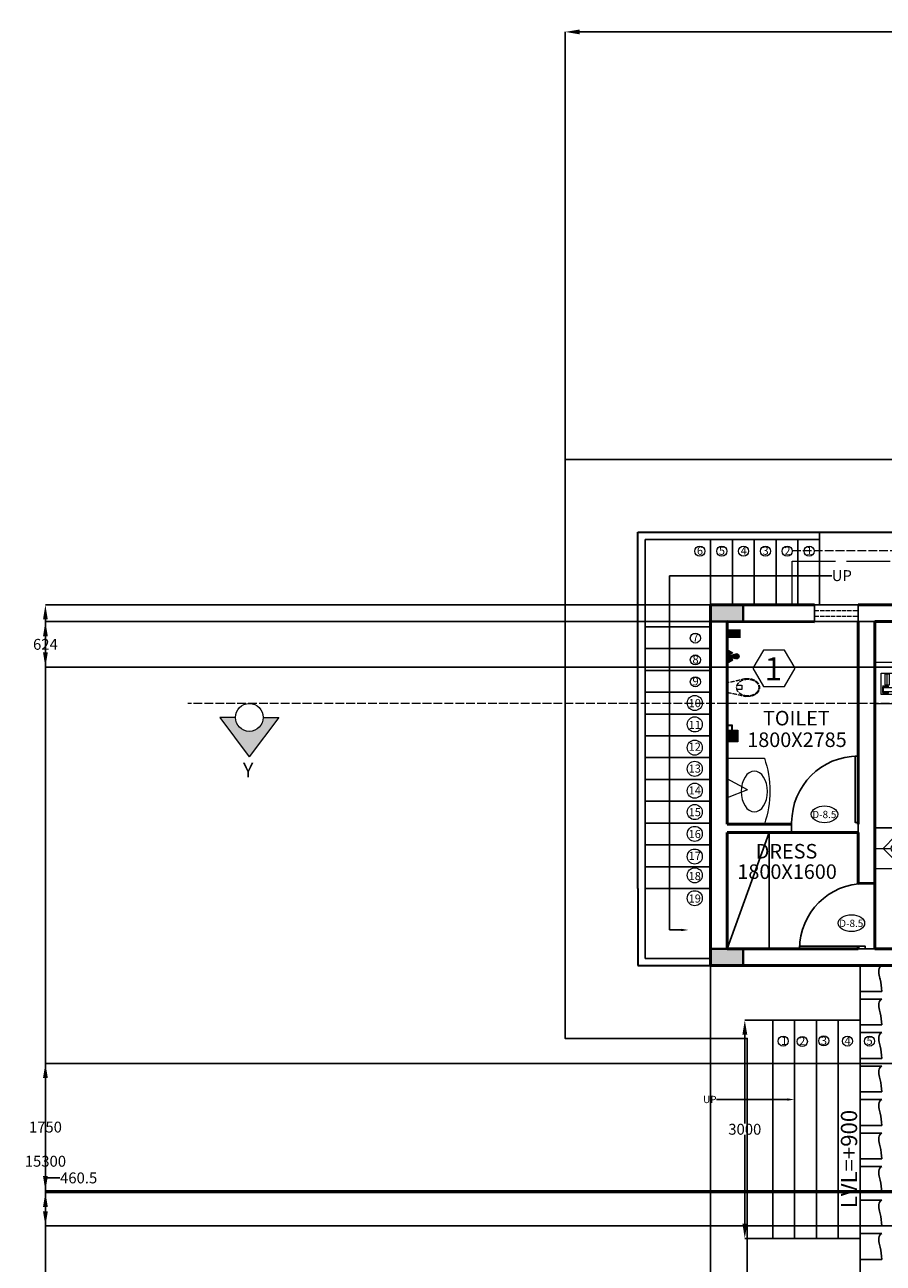
# Model space of a CAD drawing. Units: inches. Extents: x 22626 to 57351, y 2118 to 36234.
# Tile 2 of 10: x 22626 to 34432, y 19205 to 36234. Entities that reach past the tile are written whole.
import ezdxf
from ezdxf import colors
from ezdxf.entities.mleader import LeaderData, LeaderLine
from ezdxf.math import Vec2, Vec3

# ---------------------------------------------------------------- set-up
doc = ezdxf.new("R2010")
doc.units = ezdxf.units.IN
doc.header["$MEASUREMENT"] = 0
doc.linetypes.add('ACAD_ISO02W100', pattern=[15, 12, -3])
for name, color, linetype, lineweight in [('A-ANNO-DIMS', 130, 'Continuous', 18), ('A-ANNO-IDEN', 130, 'Continuous', 15), ('A-ANNO-STRS', 130, 'Continuous', 15), ('A-ANNO-SYMB', 130, 'Continuous', 18), ('A-AREA-IDEN', 130, 'Continuous', 18), ('A-COLS', 7, 'Continuous', 40), ('A-FLOR', 80, 'Continuous', 30), ('A-FLOR-CASE', 30, 'Continuous', 25), ('A-FLOR-FIXT', 30, 'Continuous', 18), ('A-FLOR-FIXT-HIDN', 30, 'ACAD_ISO02W100', 18), ('A-GLAZ-VENT', 152, 'Continuous', 25), ('A-GLAZ-VENT-HIDN', 152, 'ACAD_ISO02W100', 18), ('A-ROOF', 80, 'Continuous', 25), ('A-ROOF-OVHD', 80, 'ACAD_ISO02W100', 18), ('A-WALL', 80, 'Continuous', 50), ('DOORS', 32, 'Continuous', 25), ('FURNITURE', 30, 'Continuous', 18), ('STAIRS', 82, 'Continuous', 25)]:
    doc.layers.add(name, color=color, linetype=linetype, lineweight=lineweight)
doc.layers.add('A-SECT', color=2, linetype='ACAD_ISO02W100', lineweight=18, true_color=0xf1eb1f)
doc.styles.get("Standard").update_dxf_attribs({"font": 'arial.ttf'})
doc.dimstyles.get("Standard").update_dxf_attribs({"dimtxt": 150, "dimasz": 200, "dimexe": 0.18, "dimexo": 0.0625, "dimgap": 0.09, "dimtad": 0, "dimtih": 1, "dimtoh": 1, "dimdec": 0, "dimzin": 0, "dimdsep": 46, "dimtxsty": 'Standard', "dimcen": 0.09, "dimadec": 0, "dimazin": 0, "dimtfac": 1, "dimtdec": 0, "dimtofl": 0, "dimtmove": 0, "dimatfit": 3, "dimfxl": 1, "dimtolj": 1, "dimtzin": 0, "dimarcsym": 0})

# ---------------------------------------------------------------- blocks, each defined once
blk = doc.blocks.new('*U7')
for p, q in [((0, 0), (0, -6)), ((40, 0), (40, -6))]:
    blk.add_line(p, q)
blk.add_lwpolyline([(0, 0), (0, 40), (1.75, 40), (1.75, 0)], close=True)
blk.add_arc((0, 0), 40, 0, 90)
blk = doc.blocks.new('*D9')
at = {"layer": 'A-ANNO-DIMS', "color": 0, "lineweight": -2, "transparency": 16777216}
for p, q in [((32912, 22547), (32528, 22547)), ((32528, 22347), (32528, 21124)), ((32528, 19747), (32528, 20970)), ((32912, 19547), (32528, 19547))]:
    blk.add_line(p, q, dxfattribs=at)
at = {"layer": 'A-ANNO-DIMS', "color": 0, "transparency": 16777216}
for points in [[(32495, 22347), (32562, 22347), (32528, 22547)], [(32495, 19747), (32562, 19747), (32528, 19547)]]:
    blk.add_solid(points, dxfattribs=at)
at = {"layer": 'Defpoints', "color": 0, "transparency": 16777216}
for p in [(32912, 22547), (32528, 19547), (32912, 19547)]:
    blk.add_point(p, dxfattribs=at)
at = {"layer": 'A-ANNO-DIMS', "color": 0, "transparency": 16777216, "insert": (32528, 21047), "char_height": 150, "attachment_point": 5}
blk.add_mtext('\\A1;3000', dxfattribs=at)
blk = doc.blocks.new('Phone - Desk')
for p, q in [((-4.5, -5), (-4.5, 5)), ((-4.5, 5), (4.5, 5)), ((-4, 4.5), (-4, 2)), ((-4, 2), (-3.25, 2)), ((-3.75, 4.5), (-3.75, 2.25)), ((-1.25, 4.5), (-3.75, 4.5)), ((-3.75, 2.25), (-3.25, 2.25)), ((-3.25, 4), (-3.25, -4)), ((-3.25, 4), (-1.75, 4)), ((-1.75, -4), (-1.75, 4)), ((-1.75, 2.25), (-1.25, 2.25)), ((-1.75, 2), (-1, 2)), ((-1.25, 2.25), (-1.25, 4.5)), ((-1, 2), (-1, 4.5)), ((4, 3.5), (-0.5, 3.5)), ((-0.5, 3.5), (-0.5, 1.5)), ((-0.5, 2.5), (4, 2.5)), ((-0.5, 1.5), (4, 1.5)), ((4, 1.5), (4, 3.5)), ((4.5, 5), (4.5, -5)), ((4.5, -5), (-4.5, -5)), ((-3.75, -2.25), (-3.25, -2.25)), ((-3.75, -4.5), (-3.75, -2.25)), ((-1.25, -4.5), (-3.75, -4.5)), ((-3.25, -4), (-1.75, -4)), ((-1.75, -2.25), (-1.25, -2.25)), ((-1.25, -2.25), (-1.25, -4.5)), ((2.75, -1), (0.75, -1)), ((0.75, -1), (0.75, -4)), ((0.75, -4), (2.75, -4)), ((2.75, -4), (2.75, -1))]:
    blk.add_line(p, q)
blk = doc.blocks.new('BED')
h = blk.add_hatch()
h.set_pattern_fill('AR-B816', color=256, scale=27, angle=45)
h.paths.add_polyline_path([(36405, 26901), (36405, 25191), (35361, 25191), (35361, 24640), (36931, 24640), (36931, 25191), (36931, 27463), (36405, 27463), (35361, 27463), (35361, 26901)])
for p, q in [((35361, 26901), (35361, 27463)), ((35361, 27463), (36405, 27463)), ((36405, 27463), (36931, 27463)), ((36931, 27463), (36931, 25191)), ((35035, 26901), (35035, 26469)), ((34673, 25686), (34673, 26469)), ((35035, 26469), (34673, 26469)), ((35035, 25686), (34673, 25686)), ((34673, 25686), (35035, 25191)), ((35035, 25191), (35035, 25686)), ((34429, 24909), (34599, 25080)), ((34599, 25191), (34599, 24968)), ((34599, 25080), (34769, 24909)), ((35361, 24640), (35361, 25191)), ((36931, 25191), (36931, 24640)), ((34317, 24909), (34540, 24909)), ((34599, 24739), (34429, 24909)), ((34769, 24909), (34599, 24739)), ((34658, 24909), (34880, 24909)), ((34599, 24850), (34599, 24628)), ((36931, 24640), (35361, 24640))]:
    blk.add_line(p, q)
for points in [[(34317, 26901), (34880, 26901), (34880, 27463), (34317, 27463)], [(34317, 26901), (36405, 26901), (36405, 25191), (34317, 25191)], [(34317, 25191), (34880, 25191), (34880, 24628), (34317, 24628)]]:
    blk.add_lwpolyline(points, close=True)
blk.add_circle((34599, 24909), 59)
at = {"xscale": 32.52267765020765, "yscale": 32.52267765020765, "zscale": 32.52267765020765, "rotation": 90}
blk.add_blockref('Phone - Desk', (34567, 27173), dxfattribs=at)
blk = doc.blocks.new('WC')
at = {"ltscale": 5}
for p, q in [((307, 158), (242, 158)), ((242, 158), (242, 98)), ((242, 98), (310, 100)), ((307, 158), (307, 158))]:
    blk.add_line(p, q, dxfattribs=at)
for centre, start, end in [((781, 2286), 254.0006, 260.8285), ((781, -2036), 99.1715, 105.9994)]:
    blk.add_arc(centre, 2121, start, end, dxfattribs=at)
blk.add_ellipse((162, 125), major_axis=(152, 0), ratio=0.757128, start_param=-1.570796, end_param=4.712389, dxfattribs=at)
for points, knots in [([(196, 247), (190, 248), (184, 249), (169, 250), (159, 250), (141, 249), (132, 248), (115, 245), (106, 243), (89, 237), (81, 234), (66, 226), (59, 222), (45, 212), (39, 207), (28, 195), (23, 189), (14, 177), (10, 170), (5, 156), (3, 149), (0, 134), (0, 127), (1, 113), (2, 105), (6, 91), (9, 84), (16, 71), (20, 64), (30, 52), (35, 46), (48, 36), (55, 31), (69, 22), (77, 18), (93, 12), (101, 9), (118, 4), (127, 3), (145, 1), (153, 0), (162, 0)], [1.355035, 1.355035, 1.355035, 1.355035, 1.47179, 1.47179, 1.642812, 1.642812, 1.813835, 1.813835, 1.984858, 1.984858, 2.155881, 2.155881, 2.326904, 2.326904, 2.497927, 2.497927, 2.66895, 2.66895, 2.839973, 2.839973, 3.010996, 3.010996, 3.182019, 3.182019, 3.353042, 3.353042, 3.524065, 3.524065, 3.695088, 3.695088, 3.866111, 3.866111, 4.037134, 4.037134, 4.208157, 4.208157, 4.37918, 4.37918, 4.550203, 4.550203, 4.712389, 4.712389, 4.712389, 4.712389]), ([(162, 0), (168, 0), (174, 0), (185, 1), (191, 2), (196, 3)], [-1.5707963, -1.5707963, -1.5707963, -1.5707963, -1.4582575, -1.4582575, -1.3550165, -1.3550165, -1.3550165, -1.3550165])]:
    blk.add_open_spline(points, degree=3, knots=knots, dxfattribs=at)
blk = doc.blocks.new('VANITY-BASIN')
for p, q in [((585, 910), (75, 910)), ((306, 472), (585, 625)), ((306, 472), (585, 363))]:
    blk.add_line(p, q)
blk.add_arc((1410, 455), 1410, 161.173, 198.827)
blk.add_ellipse((213, 449), major_axis=(0, -280), ratio=0.646908)
blk = doc.blocks.new('COL-RECTANGULAR')
h = blk.add_hatch(color=256)
h.dxf.hatch_style = 1
h.paths.add_polyline_path([(0, 0), (450, 0), (450, 230), (0, 230)])
blk.add_lwpolyline([(0, 0), (0, 230), (450, 230), (450, 0)], close=True)
blk = doc.blocks.new('SECTION-HEAD')
h = blk.add_hatch(color=256)
h.dxf.hatch_style = 1
h.paths.add_polyline_path([(815, 541), (599, 541, -1), (216, 541), (0, 541), (407, 0)])
for p, q in [((216, 541), (0, 541)), ((0, 541), (407, 0)), ((815, 541), (407, 0)), ((599, 541), (815, 541))]:
    blk.add_line(p, q)
blk.add_circle((407, 541), 191)
blk = doc.blocks.new('CANOPY-EDGE-UNIT')
blk.add_lwpolyline([(0, 355), (300, 355), (300, 0), (0, 0)])
blk.add_open_spline([(0, 0), (4, 58), (10, 128), (45, 238), (49, 340), (0, 355)], degree=3, knots=[0, 0, 0, 0, 169.253843, 206.158158, 361.823024, 361.823024, 361.823024, 361.823024])
blk = doc.blocks.new('BATH-SUPPLY-FITTING')
h = blk.add_hatch(color=256)
h.dxf.hatch_style = 1
h.paths.add_polyline_path([(161, 189), (85, 141), (161, 95)])
h = blk.add_hatch(color=256)
h.dxf.hatch_style = 1
h.paths.add_polyline_path([(161, 95), (58, 125, 1.908564), (58, 64)])
h = blk.add_hatch(color=256)
h.dxf.hatch_style = 1
h.paths.add_polyline_path([(161, 95), (85, 48), (161, 0)])
for p, q in [((161, 189), (85, 141)), ((161, 95), (58, 125)), ((161, 95), (58, 64)), ((85, 141), (161, 95)), ((85, 48), (161, 95)), ((161, 0), (85, 48))]:
    blk.add_line(p, q)
blk.add_arc((37, 95), 37.1, 55.305, 304.695)
blk = doc.blocks.new('BATH-WALL-ACCESSORY')
h = blk.add_hatch(color=256)
h.dxf.hatch_style = 1
h.paths.add_polyline_path([(143, 231), (71, 231), (71, 159), (81, 159), (81, 221), (143, 221)])
h = blk.add_hatch(color=256)
h.dxf.hatch_style = 1
h.paths.add_polyline_path([(143, 159), (0, 159), (0, 0), (143, 0)])
for p, q in [((71, 159), (71, 231)), ((71, 231), (143, 231)), ((81, 221), (143, 221)), ((81, 159), (81, 221)), ((143, 159), (0, 159)), ((0, 159), (0, 0)), ((143, 159), (143, 159)), ((0, 0), (143, 0))]:
    blk.add_line(p, q)
blk = doc.blocks.new('BATH-WALL-BOX')
h = blk.add_hatch(color=256)
h.dxf.hatch_style = 1
h.paths.add_polyline_path([(182, 107), (0, 107), (0, 0), (182, 0)])
for p, q in [((0, 0), (0, 107)), ((0, 107), (182, 107)), ((182, 0), (0, 0))]:
    blk.add_line(p, q)
blk = doc.blocks.new('*D98')
at = {"layer": 'A-ANNO-DIMS', "color": 0, "lineweight": -2, "transparency": 16777216}
for p, q in [((30057, 30257), (30057, 36136)), ((30257, 36136), (39839, 36136)), ((49987, 36136), (40406, 36136)), ((50187, 30257), (50187, 36136))]:
    blk.add_line(p, q, dxfattribs=at)
at = {"layer": 'A-ANNO-DIMS', "color": 0, "transparency": 16777216}
for points in [[(30257, 36169), (30257, 36103), (30057, 36136)], [(49987, 36169), (49987, 36103), (50187, 36136)]]:
    blk.add_solid(points, dxfattribs=at)
at = {"layer": 'Defpoints', "color": 0, "transparency": 16777216}
for p in [(50187, 36136), (30057, 30257), (50187, 30257)]:
    blk.add_point(p, dxfattribs=at)
at = {"layer": 'A-ANNO-DIMS', "color": 0, "transparency": 16777216, "insert": (40122, 36136), "char_height": 150, "attachment_point": 5}
blk.add_mtext('\\A1;20130', dxfattribs=at)
blk = doc.blocks.new('*D100')
at = {"layer": 'A-ANNO-DIMS', "color": 0, "lineweight": -2, "transparency": 16777216}
for p, q in [((32057, 23297), (32057, 2216)), ((49187, 23297), (49187, 2216)), ((32257, 2216), (40347, 2216)), ((48987, 2216), (40897, 2216))]:
    blk.add_line(p, q, dxfattribs=at)
at = {"layer": 'A-ANNO-DIMS', "color": 0, "transparency": 16777216}
for points in [[(32257, 2250), (32257, 2183), (32057, 2216)], [(48987, 2250), (48987, 2183), (49187, 2216)]]:
    blk.add_solid(points, dxfattribs=at)
at = {"layer": 'Defpoints', "color": 0, "transparency": 16777216}
for p in [(32057, 23297), (49187, 23297), (49187, 2216)]:
    blk.add_point(p, dxfattribs=at)
at = {"layer": 'A-ANNO-DIMS', "color": 0, "transparency": 16777216, "insert": (40622, 2216), "char_height": 150, "attachment_point": 5}
blk.add_mtext('\\A1;17130', dxfattribs=at)
blk = doc.blocks.new('*D101')
at = {"layer": 'A-ANNO-DIMS', "color": 0, "lineweight": -2, "transparency": 16777216}
for p, q in [((31157, 28257), (22910, 28257)), ((22910, 28057), (22910, 20684)), ((22910, 13157), (22910, 20530)), ((33562, 12957), (22910, 12957))]:
    blk.add_line(p, q, dxfattribs=at)
at = {"layer": 'A-ANNO-DIMS', "color": 0, "transparency": 16777216}
for points in [[(22877, 28057), (22943, 28057), (22910, 28257)], [(22877, 13157), (22943, 13157), (22910, 12957)]]:
    blk.add_solid(points, dxfattribs=at)
at = {"layer": 'Defpoints', "color": 0, "transparency": 16777216}
for p in [(31157, 28257), (22910, 12957), (33562, 12957)]:
    blk.add_point(p, dxfattribs=at)
at = {"layer": 'A-ANNO-DIMS', "color": 0, "transparency": 16777216, "insert": (22910, 20607), "char_height": 150, "attachment_point": 5}
blk.add_mtext('\\A1;15300', dxfattribs=at)
blk = doc.blocks.new('*D107')
at = {"layer": 'A-ANNO-DIMS', "color": 0, "lineweight": -2, "transparency": 16777216}
for p, q in [((38398, 21952), (22910, 21952)), ((22910, 21752), (22910, 21154)), ((22910, 20402), (22910, 21000)), ((38398, 20202), (22910, 20202))]:
    blk.add_line(p, q, dxfattribs=at)
at = {"layer": 'A-ANNO-DIMS', "color": 0, "transparency": 16777216}
for points in [[(22877, 21752), (22943, 21752), (22910, 21952)], [(22877, 20402), (22943, 20402), (22910, 20202)]]:
    blk.add_solid(points, dxfattribs=at)
at = {"layer": 'Defpoints', "color": 0, "transparency": 16777216}
for p in [(22910, 21952), (38398, 21952), (38398, 20202)]:
    blk.add_point(p, dxfattribs=at)
at = {"layer": 'A-ANNO-DIMS', "color": 0, "transparency": 16777216, "insert": (22910, 21077), "char_height": 150, "attachment_point": 5}
blk.add_mtext('\\A1;1750', dxfattribs=at)
blk = doc.blocks.new('*D111')
at = {"layer": 'A-ANNO-DIMS', "color": 0, "lineweight": -2, "transparency": 16777216}
for p, q in [((38945, 28027), (22910, 28027)), ((22910, 27827), (22910, 27792)), ((22910, 27603), (22910, 27638)), ((38945, 27403), (22910, 27403))]:
    blk.add_line(p, q, dxfattribs=at)
at = {"layer": 'A-ANNO-DIMS', "color": 0, "transparency": 16777216}
for points in [[(22877, 27827), (22943, 27827), (22910, 28027)], [(22877, 27603), (22943, 27603), (22910, 27403)]]:
    blk.add_solid(points, dxfattribs=at)
at = {"layer": 'Defpoints', "color": 0, "transparency": 16777216}
for p in [(22910, 28027), (38945, 28027), (38945, 27403)]:
    blk.add_point(p, dxfattribs=at)
at = {"layer": 'A-ANNO-DIMS', "color": 0, "transparency": 16777216, "insert": (22910, 27715), "char_height": 150, "attachment_point": 5}
blk.add_mtext('\\A1;624', dxfattribs=at)
blk = doc.blocks.new('*D112')
at = {"layer": 'A-ANNO-DIMS', "color": 0, "lineweight": -2, "transparency": 16777216}
for p, q in [((22910, 20178), (22910, 20378)), ((22910, 20378), (23110, 20378)), ((45720, 20178), (22910, 20178)), ((22910, 19918), (22910, 19978)), ((45720, 19718), (22910, 19718))]:
    blk.add_line(p, q, dxfattribs=at)
at = {"layer": 'A-ANNO-DIMS', "color": 0, "transparency": 16777216}
for points in [[(22877, 19978), (22943, 19978), (22910, 20178)], [(22877, 19918), (22943, 19918), (22910, 19718)]]:
    blk.add_solid(points, dxfattribs=at)
at = {"layer": 'Defpoints', "color": 0, "transparency": 16777216}
for p in [(22910, 20178), (45720, 20178), (45720, 19718)]:
    blk.add_point(p, dxfattribs=at)
at = {"layer": 'A-ANNO-DIMS', "color": 0, "transparency": 16777216, "insert": (23367, 20378), "char_height": 150, "attachment_point": 5}
blk.add_mtext('\\A1;460.5', dxfattribs=at)

msp = doc.modelspace()

# ---------------------------------------------------------------- linework, layer by layer
at = {"layer": 'A-ANNO-IDEN'}
for centre in [(33624.06, 25377.62), (33994.45, 23880.56)]:
    msp.add_ellipse(centre, major_axis=(181.33, 0), ratio=0.63425497, start_param=-1.57079633, end_param=4.71238898, dxfattribs=at)
at = {"layer": 'A-ANNO-STRS'}
for centre, radius in [((31908.81, 28996.15), 69.29), ((32211.48, 28996.15), 69.29), ((32511.48, 28996.15), 69.29), ((32811.48, 28996.15), 69.29), ((33111.48, 28996.15), 69.29), ((33411.48, 28996.15), 69.29), ((31848.19, 27800.8), 69.29), ((31848.19, 27500.8), 69.29), ((31848.19, 27200.8), 69.29), ((31840.02, 26908.33), 103.8), ((31840.02, 26614.23), 103.8), ((31840.02, 26294.28), 103.8), ((31840.02, 26002.54), 103.8), ((31840.02, 25702.68), 103.8), ((31840.02, 25408.74), 103.8), ((31840.02, 25108.15), 103.8), ((31840.02, 24796.69), 103.8), ((31840.02, 24538.77), 103.8), ((31840.02, 24223.45), 103.8), ((33054.85, 22259.36), 69.29), ((33318.81, 22254.11), 69.29), ((33613.16, 22262.58), 69.29), ((33939.3, 22259.36), 69.29), ((34242.13, 22259.36), 69.29)]:
    msp.add_circle(centre, radius, dxfattribs=at)
at = {"layer": 'A-AREA-IDEN'}
msp.add_lwpolyline([(33220.33, 27385.4), (33075.13, 27636.9), (32784.72, 27636.9), (32639.51, 27385.4), (32784.72, 27133.9), (33075.13, 27133.9)], close=True, dxfattribs=at)
at = {"layer": 'A-FLOR'}
for p, q in [((31057.43, 24356.86), (31057.43, 29256.86)), ((31057.43, 29256.86), (49187.43, 29256.86)), ((31057.43, 24356.86), (31057.43, 23296.86)), ((31057.43, 23296.86), (32057.43, 23296.86))]:
    msp.add_line(p, q, dxfattribs=at)
at = {"layer": 'A-FLOR-CASE'}
for q in [(32287.43, 23526.86), (32860.98, 23526.86)]:
    msp.add_line((32860.98, 25126.86), q, dxfattribs=at)
at = {"layer": 'A-GLAZ-VENT'}
msp.add_lwpolyline([(33487.3, 28026.67), (33487.3, 28256.67), (34087.43, 28256.86), (34087.43, 28026.86)], close=True, dxfattribs=at)
at = {"layer": 'A-GLAZ-VENT-HIDN', "ltscale": 5}
for p, q in [((33487.3, 28181.86), (34087.43, 28181.86)), ((33487.3, 28101.86), (34087.43, 28101.86))]:
    msp.add_line(p, q, dxfattribs=at)
at = {"layer": 'A-ROOF'}
msp.add_line((34112.43, 23296.86), (34112.43, 18796.86), dxfattribs=at)
msp.add_lwpolyline([(43702.43, 11956.86), (43702.43, 7256.86), (37542.43, 7256.86), (37542.43, 11956.86), (32562.43, 11956.86), (32562.43, 22296.86), (30057.43, 22296.86), (30057.43, 24356.86), (30057.43, 30256.86), (39684.53, 30256.86)], dxfattribs=at)
at = {"layer": 'A-ROOF-OVHD', "ltscale": 10}
msp.add_lwpolyline([(33177.24, 29006.86), (33177.24, 29006.86), (48950.76, 29006.86), (48950.76, 28256.86)], dxfattribs=at)
at = {"layer": 'A-ROOF-OVHD', "ltscale": 50}
msp.add_lwpolyline([(33177.24, 28256.86), (33177.24, 28856.86), (48007.84, 28856.86), (48007.84, 28256.86)], dxfattribs=at)
at = {"layer": 'A-SECT', "ltscale": 10}
msp.add_line((55067.61, 26900.74), (24870.06, 26900.74), dxfattribs=at)
at = {"layer": 'A-WALL'}
for p, q in [((32057.43, 28256.86), (33487.3, 28256.67)), ((32057.43, 25011.86), (32057.43, 28256.86)), ((34087.43, 28256.86), (38047.43, 28256.86)), ((32287.43, 28026.86), (33487.3, 28026.67)), ((32287.43, 25241.86), (32287.43, 28026.86)), ((34087.43, 28026.86), (34087.43, 25241.86)), ((34317.43, 28026.86), (34317.43, 23526.86)), ((34317.43, 28026.86), (37817.43, 28026.86)), ((33172.43, 25241.86), (32287.43, 25241.86)), ((32057.43, 23296.86), (32057.43, 25126.86)), ((32287.43, 23526.86), (32287.43, 25126.86)), ((32287.43, 25126.86), (34087.43, 25126.86)), ((34087.43, 25126.86), (34087.43, 24421.83)), ((34087.43, 24424.35), (34317.43, 24429.37)), ((34087.43, 23526.86), (32287.43, 23526.86)), ((34087.43, 23566.24), (34087.43, 23526.86)), ((36907.14, 23526.86), (34317.43, 23526.86)), ((34317.43, 23296.86), (32057.43, 23296.86)), ((38047.43, 23296.86), (34317.43, 23296.86))]:
    msp.add_line(p, q, dxfattribs=at)
at = {"layer": 'STAIRS'}
for p, q in [((31157.43, 23396.86), (31157.43, 29156.71)), ((31157.43, 29156.71), (31182.33, 29156.71)), ((33557.43, 29156.71), (31182.33, 29156.71)), ((32057.43, 28256.86), (32057.43, 29156.86)), ((32357.43, 28256.86), (32357.43, 29156.86)), ((32657.43, 28256.86), (32657.43, 29156.86)), ((32957.43, 28256.86), (32957.43, 29156.86)), ((33257.43, 28256.86), (33257.43, 29156.86)), ((33557.43, 29156.71), (33557.43, 29256.86)), ((33557.43, 28256.86), (33557.43, 29156.86)), ((32057.43, 28256.86), (31157.43, 28256.86)), ((32057.43, 27956.86), (31157.43, 27956.86)), ((32057.43, 27656.86), (31157.43, 27656.86)), ((32057.43, 27356.86), (31157.43, 27356.86)), ((32057.43, 27056.86), (31157.43, 27056.86)), ((32057.43, 26756.86), (31157.43, 26756.86)), ((32057.43, 26456.86), (31157.43, 26456.86)), ((32057.43, 26156.86), (31157.43, 26156.86)), ((32057.43, 25856.86), (31157.43, 25856.86)), ((32057.43, 25556.86), (31157.43, 25556.86)), ((32057.43, 25256.86), (31157.43, 25256.86)), ((32057.43, 24956.86), (31157.43, 24956.86)), ((32057.43, 24656.86), (31157.43, 24656.86)), ((32057.43, 24356.86), (31157.43, 24356.86)), ((31157.43, 23396.86), (32057.43, 23396.86)), ((32912.43, 19546.86), (32912.43, 22546.86)), ((34112.43, 22546.86), (32912.43, 22546.86)), ((33212.43, 19546.86), (33212.43, 22546.86)), ((33512.43, 19546.86), (33512.43, 22546.86)), ((33812.43, 19546.86), (33812.43, 22546.86)), ((34112.43, 19546.86), (32912.43, 19546.86))]:
    msp.add_line(p, q, dxfattribs=at)

# ---------------------------------------------------------------- block references
at = {"layer": 'A-ANNO-SYMB'}
msp.add_blockref('SECTION-HEAD', (25307.14, 26168.47), dxfattribs=at)
at = {"layer": 'A-COLS'}
for p in [(32057.43, 28026.86), (32057.43, 23296.86)]:
    msp.add_blockref('COL-RECTANGULAR', p, dxfattribs=at)
at = {"layer": 'A-FLOR-FIXT'}
msp.add_blockref('BATH-WALL-BOX', (32287.43, 27806.86), dxfattribs=at)
at = {"layer": 'A-FLOR-FIXT', "extrusion": (0, 0, -1), "zscale": -1}
for name, p in [('BATH-SUPPLY-FITTING', (-32448.44, 27455.41)), ('BATH-WALL-ACCESSORY', (-32430.27, 26373.56)), ('VANITY-BASIN', (-32872.15, 25241.86))]:
    msp.add_blockref(name, p, dxfattribs=at)
at = {"layer": 'A-FLOR-FIXT-HIDN', "extrusion": (0, 0, -1), "zscale": -1}
msp.add_blockref('WC', (-32730.06, 26995.45), dxfattribs=at)
at = {"layer": 'A-ROOF', "extrusion": (0, 0, -1), "zscale": -1}
for p in [(-34412.43, 22941.54), (-34412.43, 22481.02), (-34412.43, 22020.5), (-34412.43, 21559.98), (-34412.43, 21099.46), (-34412.43, 20638.94), (-34412.43, 20178.42), (-34412.43, 19717.9), (-34412.43, 19257.38)]:
    msp.add_blockref('CANOPY-EDGE-UNIT', p, dxfattribs=at)
at = {"layer": 'DOORS', "xscale": -22.875, "yscale": 22.875, "zscale": 22.875}
msp.add_blockref('*U7', (34087.43, 25264.11), dxfattribs=at)
at = {"layer": 'DOORS', "xscale": 22.5, "yscale": 22.5, "zscale": 22.5, "rotation": 90.00000000000003}
msp.add_blockref('*U7', (34182.43, 23526.86), dxfattribs=at)
at = {"layer": 'FURNITURE'}
msp.add_blockref('BED', (0, 0), dxfattribs=at)

# ---------------------------------------------------------------- texts
at = {"layer": 'A-ANNO-IDEN'}
for p in [(33456.44, 25325.34), (33826.83, 23828.28)]:
    msp.add_text('D-8.5', height=100, dxfattribs=at).set_placement(p)
at = {"layer": 'A-ANNO-STRS'}
for s, height, p in [('6', 111.39, (31869.32, 28946.37)), ('5', 111.39, (32171.99, 28946.37)), ('4 ', 111.387, (32471.99, 28946.37)), ('3', 111.39, (32771.99, 28946.37)), ('2', 111.39, (33071.99, 28946.37)), ('1', 111.39, (33371.99, 28946.37)), ('7', 111.39, (31808.7, 27751.03)), ('8', 111.39, (31808.7, 27451.03)), ('9', 111.39, (31808.7, 27151.03)), ('10', 111.387, (31755.53, 26851.03)), ('11', 111.387, (31755.53, 26551.03)), ('12', 111.387, (31755.53, 26251.03)), ('13', 111.387, (31755.53, 25951.03)), ('14', 111.387, (31755.53, 25651.03)), ('15', 111.387, (31755.53, 25351.03)), ('16', 111.387, (31755.53, 25051.03)), ('17', 111.387, (31755.53, 24751.03)), ('18', 111.387, (31755.53, 24473.57)), ('19', 111.387, (31755.53, 24164.16)), ('1', 111.39, (33027.26, 22207.02)), ('2', 111.39, (33275.41, 22204.33)), ('3', 111.39, (33573.48, 22209.09)), ('4', 111.39, (33899.34, 22206.48)), ('5', 111.39, (34201.98, 22208.24))]:
    msp.add_text(s, height=height, dxfattribs=at).set_placement(p)
at = {"layer": 'A-ANNO-SYMB'}
msp.add_text('Y', height=200, dxfattribs=at).set_placement((25625.8, 25887.63))
msp.add_text('LVL=+900', height=223.502, rotation=90, dxfattribs=at).set_placement((34072.87, 19961.25))
at = {"layer": 'A-AREA-IDEN'}
for s, height, p in [('1', 318.67, (32800.36, 27218.72)), ('TOILET', 200, (32777.61, 26600.01)), ('1800X2785', 200, (32561.38, 26303.05)), ('DRESS', 200, (32678.42, 24769.84)), ('1800X1600', 200, (32425.84, 24489.13))]:
    msp.add_text(s, height=height, dxfattribs=at).set_placement(p)

# ---------------------------------------------------------------- dimensions: what is measured, and where the dimension line sits
at = {"layer": 'A-ANNO-DIMS'}
for base, p1, p2, picture, middle in [((50187.43, 36136.06), (30057.43, 30256.86), (50187.43, 30256.86), '*D98', (40122.43, 36136.06)), ((49187.43, 2216.37), (32057.43, 23296.86), (49187.43, 23296.86), '*D100', (40622.43, 2216.37))]:
    dim = msp.add_linear_dim(base=base, p1=p1, p2=p2, dimstyle='Standard', override={"dimdec": 0, "dimlfac": 1, "dimrnd": 0, "dimzin": 0, "dimdsep": 46, "dimlunit": 2}, dxfattribs=at)
    dim.commit()
    dim.dimension.update_dxf_attribs({"geometry": picture, "text_midpoint": middle})
for base, p1, p2, override, picture, middle in [((22910.07, 12956.86), (31157.43, 28256.86), (33562.43, 12956.86), {"dimdec": 0, "dimlfac": 1, "dimrnd": 0, "dimzin": 0, "dimdsep": 46, "dimlunit": 2}, '*D101', (22910.07, 20606.86)), ((22910.07, 28026.86), (38945.2, 27402.81), (38945.2, 28026.86), {"dimdec": 0, "dimlfac": 1, "dimrnd": 0, "dimzin": 0, "dimdsep": 46, "dimlunit": 2}, '*D111', (22910.07, 27714.84)), ((32528.36, 19546.86), (32912.43, 22546.86), (32912.43, 19546.86), {"dimclrd": 0, "dimclre": 0, "dimclrt": 0}, '*D9', (32528.36, 21046.86)), ((22910.07, 21952.06), (38398.28, 20202.06), (38398.28, 21952.06), {"dimdec": 0, "dimlfac": 1, "dimrnd": 0, "dimzin": 0, "dimdsep": 46, "dimlunit": 2}, '*D107', (22910.07, 21077.06)), ((22910.07, 20178.42), (45719.93, 19717.9), (45719.93, 20178.42), {"dimdec": 1, "dimlfac": 1, "dimrnd": 0, "dimzin": 0, "dimdsep": 46, "dimlunit": 2}, '*D112', (23366.83, 20378.42))]:
    dim = msp.add_linear_dim(base=base, p1=p1, p2=p2, angle=90, dimstyle='Standard', override=override, dxfattribs=at)
    dim.commit()
    dim.dimension.update_dxf_attribs({"geometry": picture, "text_midpoint": middle})

# ---------------------------------------------------------------- leaders
at = {"layer": 'A-ANNO-STRS'}
ml = msp.add_multileader_mtext('Standard', dxfattribs=at)
ml.set_content('UP', color=256)
ml.set_leader_properties()
ml.build(insert=Vec2(0, 0))
ml.multileader.update_dxf_attribs({"dogleg_length": 0.36, "arrow_head_size": 100})
ctx = ml.context
ctx.base_point, ctx.char_height, ctx.arrow_head_size, ctx.landing_gap_size, ctx.plane_origin = Vec3(33723.72, 28658.67), 150, 100, 0.09, Vec3(31752.56, 23787.33)
notes = []
notes.append((ctx, [(0, (1, 1, 0), (33723.36, 28658.67), (1, 0), 0.36, [(0, [(31752.56, 23787.33), (31492.84, 23787.33), (31492.84, 28658.67)], 0, [])])]))
ctx.mtext.insert, ctx.mtext.flow_direction = Vec3(33723.81, 28734.95), 5
ml = msp.add_multileader_mtext('Standard', dxfattribs=at)
ml.set_content('UP', color=256)
ml.set_leader_properties()
ml.build(insert=Vec2(0, 0))
ml.multileader.update_dxf_attribs({"dogleg_length": 0.36, "arrow_head_size": 100})
ctx = ml.context
ctx.base_point, ctx.char_height, ctx.arrow_head_size, ctx.landing_gap_size, ctx.plane_origin = Vec3(31962.51, 21455.79), 100, 100, 0.09, Vec3(31591, 21455.79)
ctx.text_align_type = 2
notes.append((ctx, [(0, (1, 1, 0), (32140.06, 21455.79), (-1, 0), 0.36, [(0, [(33212.43, 21455.79)], 0, [])])]))
ctx.mtext.insert, ctx.mtext.alignment, ctx.mtext.flow_direction = Vec3(32139.61, 21506.64), 3, 5
for ctx, leaders in notes:
    for number, flags, end, landing, length, lines in leaders:
        leader = LeaderData()
        leader.index, (leader.has_last_leader_line, leader.has_dogleg_vector, leader.attachment_direction) = number, flags
        leader.last_leader_point, leader.dogleg_vector, leader.dogleg_length = Vec3(end), Vec3(landing), length
        for number, points, colour, breaks in lines:
            line = LeaderLine()
            line.index, line.vertices, line.color, line.breaks = number, Vec3.list(points), colors.encode_raw_color(colour), breaks
            leader.lines.append(line)
        ctx.leaders.append(leader)

doc.saveas('drawing.dxf')
